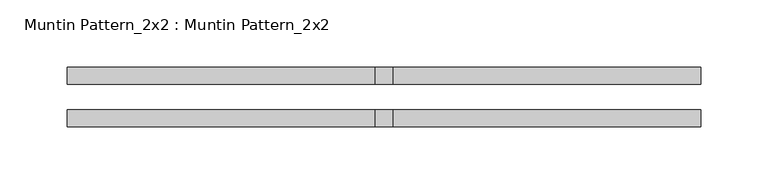
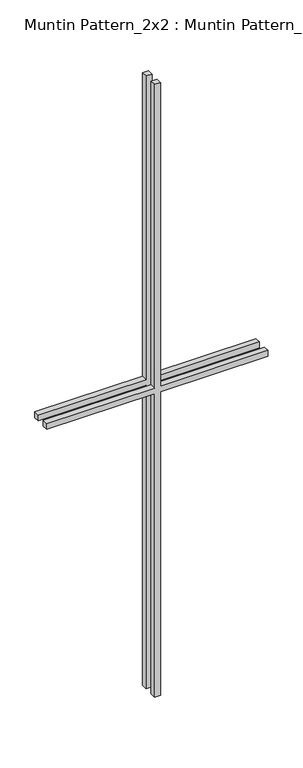
"""IFC4 building model written with IfcOpenShell, lengths in millimetres: proxy geometry, Muntin Pattern_2x2 : Muntin Pattern_2x2."""

from ifc_helpers import new_model, si_unit, frame, origin, place, context, project, spatial, polyline, outline, extrude, source, transform, mapped, element, save


def muntin_pattern_2x2_muntin_pattern_2x2_6dad3731(model_context):
    return source(origin(), model_context, "Body", "SweptSolid", [
        extrude(outline(polyline([(698.5, -6.35), (698.5, -236.5375), (685.8, -236.5375), (685.8, -6.35), (0.0, -6.35), (0.0, 6.35), (685.8, 6.35), (685.8, 236.5375), (698.5, 236.5375), (698.5, 6.35), (1384.3, 6.35), (1384.3, -6.35), (698.5, -6.35)])), frame((0.0, 9.525, 0.0), z_axis=(0.0, 1.0, 0.0), x_axis=(0.0, 0.0, 1.0)), (0.0, 0.0, 1.0), 12.7),
        extrude(outline(polyline([(698.5, -6.35), (698.5, -236.5375), (685.8, -236.5375), (685.8, -6.35), (0.0, -6.35), (0.0, 6.35), (685.8, 6.35), (685.8, 236.5375), (698.5, 236.5375), (698.5, 6.35), (1384.3, 6.35), (1384.3, -6.35), (698.5, -6.35)])), frame((0.0, -22.225, 0.0), z_axis=(0.0, 1.0, 0.0), x_axis=(0.0, 0.0, 1.0)), (0.0, 0.0, 1.0), 12.7),
    ])


if __name__ == "__main__":
    model = new_model("IFC4")
    model_context = context("Model", 3, world=origin())
    ifc_project = project(units=[si_unit("LENGTHUNIT", "METRE", prefix="MILLI")], contexts=[model_context])
    site = spatial("IfcSite", under=ifc_project)
    building = spatial("IfcBuilding", under=site)
    placement = place(None, origin())
    muntin_pattern_2x2_muntin_pattern_2x2_shape = muntin_pattern_2x2_muntin_pattern_2x2_6dad3731(model_context)
    element("IfcBuildingElementProxy", 1, Name="Muntin Pattern_2x2 : Muntin Pattern_2x2", ObjectType="Muntin Pattern_2x2 : Muntin Pattern_2x2", at=placement, inside=building, context=model_context, shape_type="MappedRepresentation", body=[
        mapped(muntin_pattern_2x2_muntin_pattern_2x2_shape, transform((0.0, 0.0, 0.0), x_axis=(1.0, 0.0, 0.0), y_axis=(0.0, 1.0, 0.0), z_axis=(0.0, 0.0, 1.0))),
    ])
    save(model, "model.ifc")

# Revit data of these elements
# Type "Muntin Pattern_2x2 : Muntin Pattern_2x2"
#   Width [instance default] = 4' - 0"
#   Thickness = 0' - 0 1/2"
#   Height [instance default] = 4' - 0"
#   Distance = 0' - 0 3/4"
#   Interior Material [instance default] = none
#   Exterior Material [instance default] = none
#   Default Elevation = 0
# Element 1 (IfcBuildingElementProxy, "Muntin Pattern_2x2 : Muntin Pattern_2x2")
#   Width = 1' - 6 5/8"
#   Height = 4' - 6 1/2"
#   Interior Material = Wood - Stained
#   Exterior Material = BLACK MATERIAL
#   Materials on its faces: "BLACK MATERIAL", "Wood - Stained"
# Materials
#   "BLACK MATERIAL": class "Generic", colour RGB 120 120 120, transparency 0, Cost = 0
#   "Wood - Stained": class "Wood", colour RGB 224 178 126, transparency 0, Cost = 0
